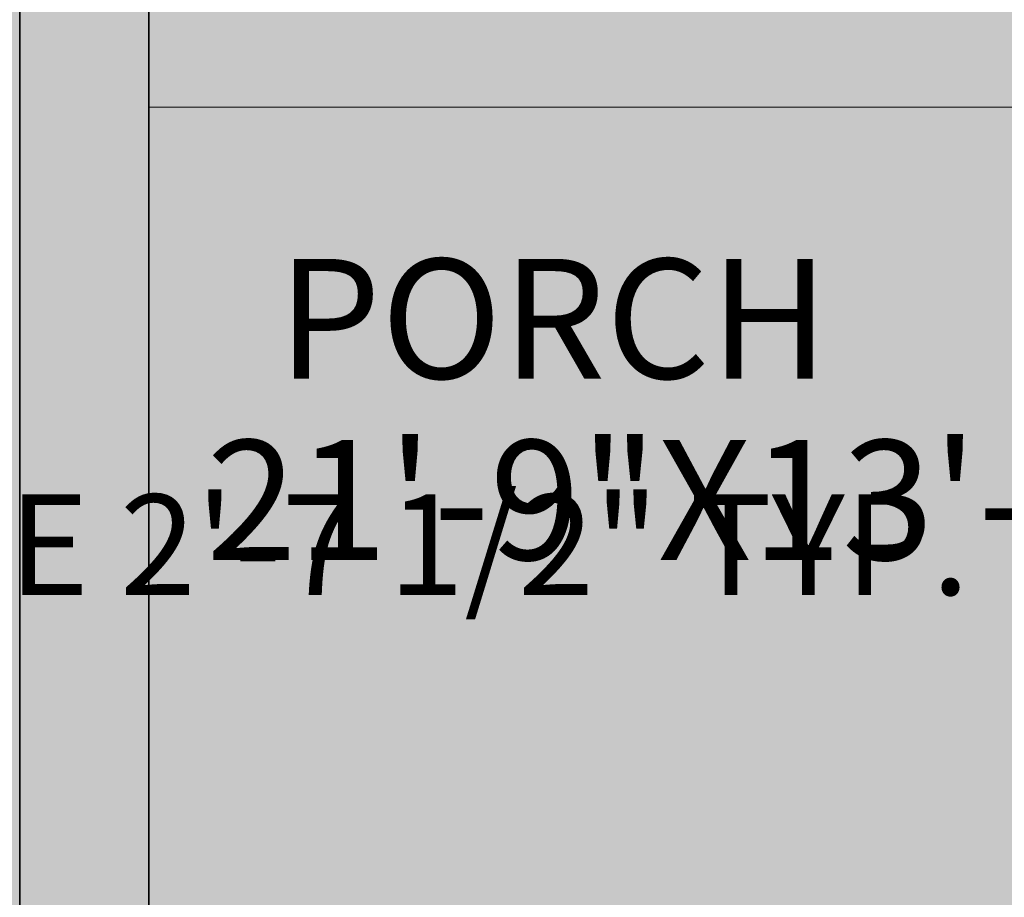
# Model space of a CAD drawing. Units: inches. Extents: x 1884 to 2398, y 474 to 1488.
# Tile 14 of 39: x 2118 to 2186, y 699 to 761. Entities that reach past the tile are written whole.
import ezdxf

# ---------------------------------------------------------------- set-up
doc = ezdxf.new("R2010")
doc.units = ezdxf.units.IN
doc.header["$MEASUREMENT"] = 0
for name, color, linetype, lineweight in [('A-ANNO-DIMS', 2, 'Continuous', 18), ('A-AREA-IDEN', 7, 'Continuous', 18), ('A-FLOR-PATT', 254, 'Continuous', 13), ('A-FLOR-STRS', 7, 'Continuous', 20), ('A-WALL-PATT', 250, 'Continuous', 13), ('walls', 7, 'Continuous', 35)]:
    doc.layers.add(name, color=color, linetype=linetype, lineweight=lineweight)
doc.layers.add('A-FLOR-STRS-PATT', color=251, linetype='Continuous', lineweight=13, true_color=0x636466)
doc.layers.add('L-PVMT-PATT', color=9, linetype='Continuous', lineweight=13, true_color=0xc7c8ca)
doc.styles.get("Standard").update_dxf_attribs({"font": 'arial.ttf'})
doc.dimstyles.get("Standard").update_dxf_attribs({"dimtxt": 7, "dimasz": 0.18, "dimexe": 0.18, "dimexo": 0.0625, "dimgap": 0.09, "dimtad": 0, "dimtih": 1, "dimtoh": 1, "dimzin": 0, "dimdsep": 46, "dimlunit": 3, "dimtxsty": 'Standard', "dimcen": 0.09, "dimadec": 0, "dimazin": 0, "dimtfac": 1, "dimtofl": 0, "dimtmove": 0, "dimatfit": 3, "dimfxl": 1, "dimtolj": 1, "dimtzin": 0, "dimarcsym": 0})

# ---------------------------------------------------------------- blocks, each defined once
blk = doc.blocks.new('*D33')
at = {"layer": 'A-ANNO-DIMS', "color": 0, "lineweight": -2, "transparency": 16777216}
for p, q in [((2021.148, 719.326), (2021.148, 724.135)), ((2021.328, 723.955), (2052.246, 723.955)), ((2052.426, 719.326), (2052.426, 724.135)), ((2052.426, 723.955), (2052.606, 723.955))]:
    blk.add_line(p, q, dxfattribs=at)
at = {"layer": 'A-ANNO-DIMS', "color": 0, "lineweight": 100, "transparency": 16777216}
for points in [[(2021.328, 723.985), (2021.328, 723.925), (2021.148, 723.955)], [(2052.246, 723.985), (2052.246, 723.925), (2052.426, 723.955)]]:
    blk.add_solid(points, dxfattribs=at)
at = {"layer": 'Defpoints', "color": 0, "lineweight": 100, "transparency": 16777216}
for p in [(2052.426, 723.955), (2021.148, 719.264), (2052.426, 719.264)]:
    blk.add_point(p, dxfattribs=at)
at = {"layer": 'A-ANNO-DIMS', "color": 0, "transparency": 16777216, "insert": (2120.182, 723.955), "char_height": 7, "attachment_point": 5}
blk.add_mtext('\\A1;COFFEE TABLE 2\'-7 1/2" TYP.', dxfattribs=at)

msp = doc.modelspace()

# ---------------------------------------------------------------- hatches: boundary and pattern name
at = {"layer": 'A-FLOR-PATT'}
h = msp.add_hatch(color=256, dxfattribs=at)
h.dxf.hatch_style = 1
h.paths.add_polyline_path([(2117.529, 815.801), (2126.529, 815.801), (2126.529, 880.382), (2117.529, 880.382), (2117.529, 892.385), (1961.529, 892.385), (1961.529, 756.915), (1964.529, 756.915), (1964.529, 759.915), (1995.529, 759.915), (1995.529, 753.915), (1972.862, 753.915), (1967.529, 756.915), (1967.529, 654.915), (1972.862, 657.915), (1995.529, 657.915), (1995.529, 651.915), (1964.529, 651.915), (1964.529, 654.915), (1961.529, 654.915), (1961.529, 640.385), (2117.529, 640.385), (2117.529, 646.578), (2126.529, 646.578), (2126.529, 676.183), (2117.529, 676.183)])
h.paths.add_polyline_path([(2012.246, 808.929), (2012.05, 810.185), (2032.542, 810.185), (2032.346, 808.929)], flags=16)
h.paths.add_polyline_path([(2010.381, 820.864), (1994.658, 820.864), (1994.658, 831.561), (1984.608, 833.132), (1984.608, 853.821), (1994.658, 855.391), (1994.658, 866.089), (2010.381, 866.089), (2011.951, 876.139), (2032.64, 876.139), (2034.211, 866.089), (2045.556, 866.089), (2047.127, 876.139), (2067.816, 876.139), (2069.386, 866.089), (2085.109, 866.089), (2085.109, 855.391), (2095.159, 853.821), (2095.159, 833.132), (2085.109, 831.561), (2085.109, 820.864), (2069.386, 820.864), (2067.816, 810.814), (2047.127, 810.814), (2045.556, 820.864), (2034.211, 820.864), (2032.64, 810.814), (2011.951, 810.814)], flags=16)
h.paths.add_polyline_path([(1982.724, 833.426), (1982.724, 853.526), (1983.98, 853.723), (1983.98, 833.23)], flags=16)
h.paths.add_polyline_path([(1994.529, 753.54), (1994.529, 658.29), (1973.529, 658.29), (1973.529, 753.54)], flags=16)
h.paths.add_polyline_path([(2084.486, 843.527), (2084.592, 843.502), (2084.681, 843.487), (2084.813, 843.477), (2084.913, 843.477), (2084.669, 843.482), (2084.336, 843.565), (2084.116, 843.617), (2083.8, 843.686), (2083.105, 843.827), (2082.836, 843.874), (2083.604, 843.729), (2084.206, 843.597)], flags=0)
h.paths.add_polyline_path([(2047.421, 808.929), (2047.225, 810.185), (2067.718, 810.185), (2067.521, 808.929)], flags=16)
h.paths.add_polyline_path([(2066.01, 849.505), (2066.429, 849.687), (2066.798, 849.882), (2067.129, 850.085), (2067.43, 850.293), (2067.711, 850.502), (2068.176, 850.856), (2068.689, 851.205), (2069.305, 851.531), (2070.015, 851.784), (2070.844, 851.944), (2071.081, 851.956), (2070.629, 851.902), (2070.212, 851.822), (2069.827, 851.717), (2069.471, 851.59), (2069.139, 851.443), (2068.828, 851.279), (2068.534, 851.1), (2068.254, 850.909), (2067.983, 850.709), (2067.502, 850.343), (2066.951, 849.962), (2066.224, 849.579)], flags=0)
h.paths.add_polyline_path([(2059.423, 853.221), (2059.827, 853.278), (2060.171, 853.358), (2060.465, 853.463), (2060.714, 853.589), (2060.926, 853.736), (2061.107, 853.902), (2061.258, 854.086), (2061.377, 854.284), (2061.462, 854.495), (2061.514, 854.715), (2061.53, 854.943), (2061.508, 855.176), (2061.449, 855.411), (2061.352, 855.646), (2061.224, 855.882), (2061.07, 856.117), (2060.9, 856.353), (2060.719, 856.588), (2060.406, 856.993), (2060.103, 857.424), (2059.858, 857.888), (2059.691, 858.467), (2059.836, 859.091), (2060.305, 859.532), (2060.844, 859.798), (2061.513, 859.935), (2062.253, 859.905), (2062.483, 859.849), (2062.078, 859.912), (2061.695, 859.928), (2061.336, 859.899), (2061.005, 859.831), (2060.703, 859.729), (2060.437, 859.597), (2060.208, 859.441), (2060.021, 859.265), (2059.879, 859.075), (2059.785, 858.874), (2059.737, 858.664), (2059.73, 858.447), (2059.761, 858.224), (2059.827, 857.996), (2059.923, 857.765), (2060.047, 857.53), (2060.193, 857.295), (2060.359, 857.06), (2060.537, 856.824), (2060.867, 856.399), (2061.171, 855.978), (2061.422, 855.518), (2061.567, 854.943), (2061.41, 854.272), (2060.947, 853.707), (2060.335, 853.397), (2059.649, 853.236)], flags=0)
h.paths.add_polyline_path([(2050.778, 859.745), (2051.07, 859.87), (2051.295, 860.017), (2051.467, 860.183), (2051.594, 860.365), (2051.679, 860.56), (2051.726, 860.763), (2051.739, 860.971), (2051.722, 861.18), (2051.677, 861.387), (2051.609, 861.587), (2051.521, 861.779), (2051.421, 861.962), (2051.312, 862.138), (2051.203, 862.307), (2050.966, 862.68), (2050.793, 863.193), (2051.021, 863.699), (2051.483, 864.018), (2052.09, 864.138), (2052.773, 864.157), (2053.007, 864.142), (2052.603, 864.152), (2052.258, 864.142), (2051.965, 864.113), (2051.716, 864.064), (2051.504, 863.995), (2051.322, 863.907), (2051.17, 863.802), (2051.048, 863.682), (2050.954, 863.55), (2050.891, 863.408), (2050.856, 863.259), (2050.851, 863.105), (2050.876, 862.948), (2050.929, 862.791), (2051.005, 862.633), (2051.098, 862.472), (2051.203, 862.307), (2051.312, 862.138), (2051.556, 861.742), (2051.751, 861.167), (2051.712, 860.535), (2051.398, 860.085), (2050.949, 859.79)], flags=0)
h.paths.add_polyline_path([(2022.768, 719.264), (2050.461, 719.264), (2050.461, 717.226), (2052.426, 717.226), (2052.426, 715.033), (2050.461, 715.033), (2050.461, 703.738), (2022.768, 703.738)], flags=16)
h.paths.add_polyline_path([(2012.246, 878.023), (2032.346, 878.023), (2032.542, 876.767), (2012.05, 876.767)], flags=16)
h.paths.add_polyline_path([(2035.324, 713.103), (2035.342, 713.294), (2035.192, 713.202)], flags=0)
h.paths.add_polyline_path([(2036.484, 711.63), (2036.583, 711.849), (2036.39, 711.898)], flags=0)
h.paths.add_polyline_path([(2036.074, 712.744), (2035.993, 712.481), (2035.724, 712.516), (2035.794, 712.726)], flags=0)
h.paths.add_polyline_path([(2035.846, 710.909), (2035.753, 710.958), (2035.702, 710.88)], flags=0)
h.paths.add_polyline_path([(2037.818, 712.019), (2037.948, 712.06), (2037.987, 712.161), (2037.815, 712.02)], flags=0)
h.paths.add_polyline_path([(2038.451, 709.517), (2038.464, 709.428), (2038.586, 709.442)], flags=0)
h.paths.add_polyline_path([(2037.805, 709.806), (2037.818, 709.807), (2037.804, 709.823)], flags=0)
h.paths.add_polyline_path([(2036.7, 711.245), (2036.698, 711.236), (2036.813, 711.211)], flags=0)
h.paths.add_polyline_path([(2035.928, 708.897), (2035.668, 708.871), (2035.706, 708.667)], flags=0)
h.paths.add_polyline_path([(2036.414, 710.976), (2035.932, 709.859), (2036.792, 710.484), (2036.5, 710.934)], flags=0)
h.paths.add_polyline_path([(2038.298, 712.115), (2038.499, 712.058), (2038.612, 712.269), (2038.39, 712.332)], flags=0)
h.paths.add_polyline_path([(2047.421, 878.023), (2067.521, 878.023), (2067.718, 876.767), (2047.225, 876.767)], flags=16)
h.paths.add_polyline_path([(2049.647, 705.093, -1), (2048.845, 705.093, -1)], flags=0)
h.paths.add_polyline_path([(2095.787, 853.723), (2097.043, 853.526), (2097.043, 833.426), (2095.787, 833.23)], flags=16)
h.paths.add_polyline_path([(2110.739, 745.339), (2111.75, 745.339, -0.064042), (2113.267, 742.92), (2113.267, 732.192), (2113.526, 732.192, -0.414214), (2114.278, 731.439), (2114.278, 716.764, -0.414214), (2113.526, 716.011), (2113.267, 716.011), (2113.267, 705.284, -0.064042), (2111.75, 702.864), (2110.739, 702.864), (2110.739, 716.011), (2109.469, 716.011, -0.414214), (2108.716, 716.764), (2108.716, 731.439, -0.414214), (2109.469, 732.192), (2110.739, 732.192)], flags=16)
h.paths.add_polyline_path([(1998.045, 668.909), (2002.449, 668.909), (2002.449, 652.273), (2002.724, 652.763), (2002.724, 668.175), (2019.972, 668.175), (2019.972, 652.763), (2020.247, 652.273), (2020.247, 668.909), (2024.651, 668.909), (2029.055, 668.909), (2029.055, 652.273), (2029.33, 652.763), (2029.33, 668.175), (2046.578, 668.175), (2046.578, 652.763), (2046.853, 652.273), (2046.853, 668.909), (2051.257, 668.909), (2051.257, 646.157), (2049.055, 646.157), (2049.055, 643.955), (2026.853, 643.955), (2026.853, 646.157), (2024.651, 646.157), (2022.449, 646.157), (2022.449, 643.955), (2000.247, 643.955), (2000.247, 646.157), (1998.045, 646.157)], flags=16)
h.paths.add_polyline_path([(2342.529, 1247.885), (2265.892, 1247.885), (2230.029, 1247.885), (2209.755, 1247.885), (2168.6, 1247.885), (2168.6, 1104.929), (2158.029, 1104.929), (2158.029, 1079.411), (2168.6, 1079.411), (2168.6, 1062.466), (2342.529, 1062.466), (2342.529, 1093.809)])
h.paths.add_polyline_path([(2215.03, 1153.876), (2215.03, 1164.739), (2187.559, 1164.739), (2187.442, 1152.641), (2173.568, 1152.641), (2173.684, 1164.739), (2173.684, 1218.739), (2173.801, 1230.837), (2187.675, 1230.837), (2187.559, 1218.739), (2215.03, 1218.739), (2215.03, 1225.879), (2245.053, 1225.879), (2245.053, 1153.876)], flags=16)
h.paths.add_polyline_path([(2192.147, 1164.797), (2184.963, 1174.54), (2184.915, 1174.54), (2176.755, 1174.54), (2176.755, 1190.363), (2184.915, 1190.363), (2184.915, 1196.819), (2176.755, 1196.819), (2176.755, 1212.641), (2184.915, 1212.641), (2184.915, 1174.606), (2184.963, 1174.54), (2192.147, 1174.54)], flags=0)
h.paths.add_polyline_path([(2184.971, 1158.364, -1), (2176.039, 1158.364, -1)], flags=0)
h.paths.add_polyline_path([(2335.555, 1161.985), (2335.555, 1175.132), (2334.285, 1175.132, -0.414214), (2333.533, 1175.885), (2333.533, 1190.56, -0.414214), (2334.285, 1191.313), (2335.555, 1191.313), (2335.555, 1204.46), (2336.567, 1204.46, -0.064042), (2338.083, 1202.04), (2338.083, 1191.313), (2338.342, 1191.313, -0.414214), (2339.095, 1190.56), (2339.095, 1175.885, -0.414214), (2338.342, 1175.132), (2338.083, 1175.132), (2338.083, 1164.405, -0.064042), (2336.567, 1161.985)], flags=16)
h.paths.add_polyline_path([(2176.155, 1224.462, -1), (2185.087, 1224.462, -1)], flags=0)
h.paths.add_polyline_path([(2158.029, 1276.197), (2158.029, 1322.885), (2148.233, 1322.885), (2092.029, 1322.885), (1961.529, 1322.885), (1961.529, 1166.885), (2116.005, 1166.885), (2116.005, 1157.885), (2152.638, 1157.885), (2152.638, 1166.885), (2158.029, 1166.885)])
h.paths.add_polyline_path([(2006.352, 1204.245), (2006.352, 1215.108), (1978.881, 1215.108), (1978.764, 1203.01), (1964.89, 1203.01), (1965.006, 1215.108), (1965.006, 1269.108), (1965.123, 1281.207), (1978.997, 1281.207), (1978.881, 1269.108), (2006.352, 1269.108), (2006.352, 1276.248), (2036.375, 1276.248), (2036.375, 1204.245)], flags=16)
h.paths.add_polyline_path([(1983.469, 1215.166), (1976.285, 1224.909), (1976.237, 1224.909), (1968.077, 1224.909), (1968.077, 1240.732), (1976.237, 1240.732), (1976.237, 1247.188), (1968.077, 1247.188), (1968.077, 1263.011), (1976.237, 1263.011), (1976.237, 1224.975), (1976.285, 1224.909), (1983.469, 1224.909)], flags=0)
h.paths.add_polyline_path([(1976.293, 1208.733, -1), (1967.361, 1208.733, -1)], flags=0)
h.paths.add_polyline_path([(1967.477, 1274.832, -1), (1976.41, 1274.832, -1)], flags=0)
h.paths.add_polyline_path([(2152.587, 1223.485), (2152.587, 1236.632), (2151.317, 1236.632, -0.414214), (2150.564, 1237.385), (2150.564, 1252.06, -0.414214), (2151.317, 1252.813), (2152.587, 1252.813), (2152.587, 1265.959), (2153.598, 1265.959, -0.064042), (2155.115, 1263.54), (2155.115, 1252.813), (2155.374, 1252.813, -0.414214), (2156.126, 1252.06), (2156.126, 1237.385, -0.414214), (2155.374, 1236.632), (2155.115, 1236.632), (2155.115, 1225.904, -0.064042), (2153.598, 1223.485)], flags=16)
h.paths.add_polyline_path([(2250.676, 1161.101), (2322.077, 1161.101), (2322.077, 1173.886), (2250.676, 1173.886)], flags=24)
h.paths.add_polyline_path([(2255.61, 1173.712), (2320.136, 1173.712), (2320.136, 1186.659), (2255.61, 1186.659)], flags=24)
h.paths.add_polyline_path([(2053.687, 1230.837), (2125.089, 1230.837), (2125.089, 1243.622), (2053.687, 1243.622)], flags=24)
h.paths.add_polyline_path([(2058.622, 1243.448), (2123.147, 1243.448), (2123.147, 1256.395), (2058.622, 1256.395)], flags=24)
at = {"layer": 'A-FLOR-STRS-PATT'}
h = msp.add_hatch(color=256, dxfattribs=at)
h.dxf.hatch_style = 1
h.paths.add_polyline_path([(2238.447, 769.966), (2198.529, 769.966), (2193.526, 769.966), (2132.515, 769.966), (2126.529, 769.966), (2126.529, 762.15), (2238.447, 762.15)])
h.paths.add_polyline_path([(2238.447, 762.15), (2126.529, 762.15), (2126.529, 754.445), (2238.447, 754.445)])
at = {"layer": 'A-WALL-PATT'}
h = msp.add_hatch(color=256, dxfattribs=at)
h.dxf.hatch_style = 1
h.paths.add_polyline_path([(2351.529, 837.963), (2342.529, 837.963), (2342.529, 813.478), (2351.529, 813.478)])
h.paths.add_polyline_path([(2351.529, 782.175), (2342.529, 782.175), (2342.529, 778.966), (2238.447, 778.966), (2238.447, 769.966), (2351.529, 769.966)])
h.paths.add_polyline_path([(2351.529, 914.773), (2342.529, 914.773), (2342.529, 901.966), (2222.529, 901.966), (2222.529, 908.236), (2213.529, 908.236), (2213.529, 901.966), (2198.529, 901.966), (2198.529, 892.966), (2198.529, 815.857), (2203.029, 815.857), (2203.029, 892.966), (2342.529, 892.966), (2342.529, 869.555), (2346.047, 869.555), (2351.529, 869.555), (2351.529, 880.385)])
h.paths.add_polyline_path([(2208.948, 778.966), (2203.029, 778.966), (2203.029, 782.647), (2198.529, 782.647), (2198.529, 779.109), (2193.526, 779.109), (2193.526, 769.966), (2198.529, 769.966), (2208.948, 769.966)])
h.paths.add_polyline_path([(2126.529, 815.801), (2117.529, 815.801), (2117.529, 676.183), (2126.529, 676.183), (2126.529, 769.966), (2132.515, 769.966), (2132.515, 778.664), (2126.529, 778.664)])
h.paths.add_polyline_path([(2135.996, 901.385), (2009.529, 901.385), (2009.529, 929.544), (2000.529, 929.544), (2000.529, 892.385), (2117.529, 892.385), (2117.529, 880.382), (2126.529, 880.382), (2126.529, 892.385), (2135.996, 892.385)])
h.paths.add_polyline_path([(2198.529, 901.385), (2185.2, 901.385), (2185.2, 892.385), (2198.529, 892.385), (2198.529, 892.966)])
h.paths.add_polyline_path([(1961.529, 892.385), (1965.143, 892.385), (1965.143, 901.385), (1952.529, 901.385), (1952.529, 604.13), (1961.529, 604.13), (1961.529, 631.385), (1988.002, 631.385), (1988.002, 640.385), (1961.529, 640.385)])
h.paths.add_polyline_path([(1955.529, 604.13), (1952.529, 604.13), (1952.529, 530.885), (2126.529, 530.885), (2126.529, 533.885), (1955.529, 533.885)])
h.paths.add_polyline_path([(2396.529, 604.13), (2393.529, 604.13), (2393.529, 533.885), (2126.529, 533.885), (2126.529, 530.885), (2396.529, 530.885)])
h.paths.add_polyline_path([(2396.529, 779.322), (2387.529, 779.322), (2387.529, 604.13), (2396.529, 604.13)])
at = {"layer": 'L-PVMT-PATT'}
h = msp.add_hatch(color=256, dxfattribs=at)
h.dxf.hatch_style = 1
h.paths.add_polyline_path([(2387.529, 769.966), (2351.529, 769.966), (2238.447, 769.966), (2238.447, 762.15), (2238.447, 754.445), (2126.529, 754.445), (2126.529, 676.183), (2134.868, 676.183), (2142.673, 676.183), (2142.673, 646.578), (2134.868, 646.578), (2126.529, 646.578), (2126.529, 640.17), (2387.529, 640.17)])
h.paths.add_polyline_path([(2387.529, 631.385), (2303.086, 631.385), (2303.086, 615.671), (2387.529, 615.671)])
h.paths.add_polyline_path([(2387.529, 640.17), (2126.529, 640.17), (2126.529, 631.385), (2387.529, 631.385)])
h.paths.add_polyline_path([(2393.529, 604.13), (2387.529, 604.13), (2387.529, 615.671), (2303.086, 615.671), (2303.086, 607.943), (2249.649, 607.943), (2126.529, 607.943), (2126.529, 533.885), (2393.529, 533.885)])
h.paths.add_polyline_path([(2257.825, 611.008), (2257.83, 611.337), (2257.915, 616.493), (2258.021, 621.805), (2258.146, 627.274), (2258.252, 631.385), (2126.529, 631.385), (2126.529, 611.008)])
h.paths.add_polyline_path([(2258.892, 611.285), (2258.888, 611.008), (2300.247, 611.008), (2300.247, 631.385), (2259.314, 631.385), (2259.206, 627.173), (2259.081, 621.72), (2258.976, 616.424)])

# ---------------------------------------------------------------- linework, layer by layer
at = {"layer": 'A-FLOR-STRS'}
msp.add_line((2126.529, 754.445), (2238.447, 754.445), dxfattribs=at)
at = {"layer": 'walls'}
for p, q in [((2117.529, 676.183), (2117.529, 815.801)), ((2126.529, 530.885), (2126.529, 769.966))]:
    msp.add_line(p, q, dxfattribs=at)

# ---------------------------------------------------------------- texts
at = {"layer": 'A-AREA-IDEN'}
for s, height, p in [('PORCH', 8.3413, (2135.495, 735.527)), ('21\'-9"X13\'-9"', 8.34125, (2130.533, 722.895))]:
    msp.add_text(s, height=height, dxfattribs=at).set_placement(p)

# ---------------------------------------------------------------- dimensions: what is measured, and where the dimension line sits
at = {"layer": 'A-ANNO-DIMS'}
dim = msp.add_linear_dim(base=(2052.426, 723.955), p1=(2021.148, 719.264), p2=(2052.426, 719.264), text='COFFEE TABLE <> TYP.', dimstyle='Standard', override={"dimdec": 1, "dimlfac": 1, "dimrnd": 0, "dimzin": 1, "dimdsep": 46, "dimlunit": 4, "dimfrac": 2}, dxfattribs=at)
dim.commit()
dim.dimension.update_dxf_attribs({"geometry": '*D33', "text_midpoint": (2120.182, 723.955)})

doc.saveas('drawing.dxf')
